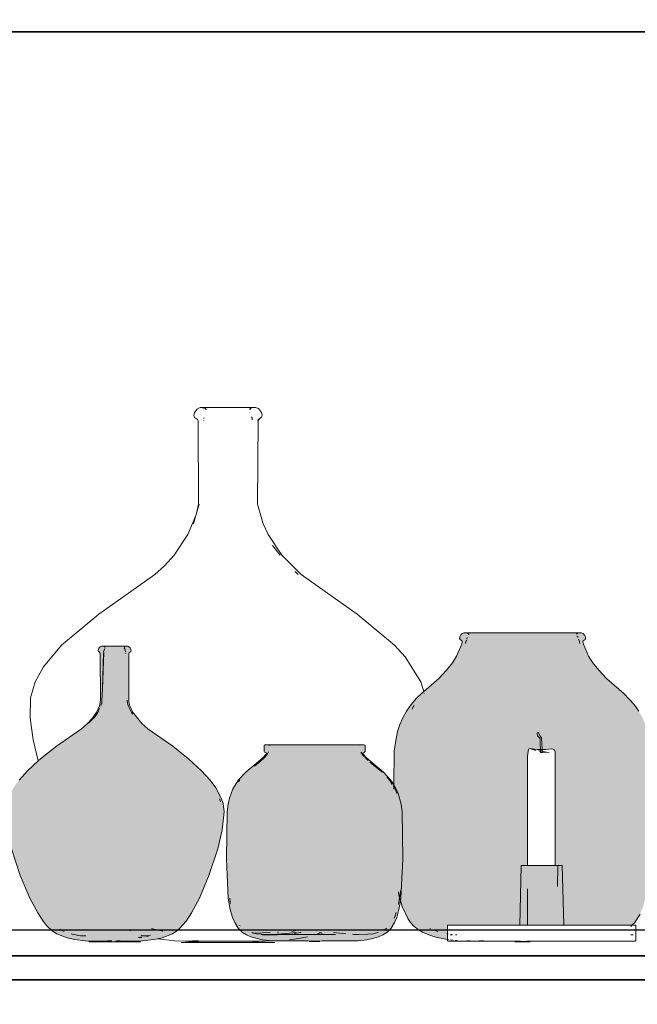
# Model space of a CAD drawing. Units: millimetres. Extents: x 446512 to 447461, y 70395 to 70610.
# Tile 16 of 39: x 446712 to 446725, y 70473 to 70493. Entities that reach past the tile are written whole.
import ezdxf

# ---------------------------------------------------------------- set-up
doc = ezdxf.new("R2010")
doc.units = ezdxf.units.MM
for name, color, linetype, lineweight in [('A-ANNO-DIMS', 2, 'Continuous', 18), ('A-FURN', 7, 'Continuous', 35), ('A-FURN-DECO', 8, 'Continuous', 13), ('A-FURN-PATT', 38, 'Continuous', 13)]:
    doc.layers.add(name, color=color, linetype=linetype, lineweight=lineweight)
doc.styles.get("Standard").update_dxf_attribs({"font": 'arial.ttf'})
doc.dimstyles.get("Standard").update_dxf_attribs({"dimtxt": 0.18, "dimasz": 0.18, "dimexe": 0.18, "dimexo": 0.0625, "dimgap": 0.09, "dimtad": 0, "dimtih": 1, "dimtoh": 1, "dimdec": 4, "dimzin": 0, "dimdsep": 46, "dimtxsty": 'Standard', "dimcen": 0.09, "dimadec": 0, "dimazin": 0, "dimtfac": 1, "dimtdec": 4, "dimtofl": 0, "dimtmove": 0, "dimatfit": 3, "dimfxl": 1, "dimtolj": 1, "dimtzin": 0, "dimarcsym": 0})

# ---------------------------------------------------------------- blocks, each defined once
blk = doc.blocks.new('*D32')
at = {"layer": 'A-ANNO-DIMS', "color": 0, "lineweight": -2, "transparency": 16777216}
for p, q in [((446730.76, 70474.405), (446678.043, 70474.405)), ((446678.223, 70474.225), (446678.223, 70474.075)), ((446678.223, 70473.562), (446678.223, 70473.711)), ((446728.946, 70473.382), (446678.043, 70473.382))]:
    blk.add_line(p, q, dxfattribs=at)
at = {"layer": 'A-ANNO-DIMS', "color": 0, "transparency": 16777216}
for points in [[(446678.193, 70474.225), (446678.253, 70474.225), (446678.223, 70474.405)], [(446678.193, 70473.562), (446678.253, 70473.562), (446678.223, 70473.382)]]:
    blk.add_solid(points, dxfattribs=at)
at = {"layer": 'Defpoints', "color": 0, "transparency": 16777216}
for p in [(446730.822, 70474.405), (446678.223, 70473.382), (446729.008, 70473.382)]:
    blk.add_point(p, dxfattribs=at)
at = {"layer": 'A-ANNO-DIMS', "color": 0, "transparency": 16777216, "insert": (446678.223, 70473.893), "char_height": 0.18, "attachment_point": 5}
blk.add_mtext('\\A1;1.02', dxfattribs=at)

msp = doc.modelspace()

# ---------------------------------------------------------------- hatches: boundary and pattern name
at = {"layer": 'A-FURN-PATT'}
h = msp.add_hatch(color=256, dxfattribs=at)
h.dxf.hatch_style = 1
h.paths.add_polyline_path([(446703.5722, 70477.5476), (446703.5295, 70477.5904), (446703.508, 70477.5904), (446703.383, 70477.6041), (446703.3062, 70477.6039), (446702.8621, 70477.6193), (446702.7177, 70477.6193), (446702.6174, 70477.6163), (446702.576, 70477.615), (446702.5757, 70477.6192), (446702.3373, 70477.6192), (446701.7238, 70477.5898), (446701.6039, 70477.5792), (446701.5612, 70477.5357), (446701.547, 70474.1653), (446703.5225, 70474.1653), (446703.5865, 70474.1653), (446703.5861, 70474.2632), (446703.5852, 70474.4594)])
h.paths.add_polyline_path([(446715.9764, 70475.5286), (446716.1565, 70476.0766), (446716.2492, 70476.4728), (446716.2873, 70476.8422), (446716.2666, 70477.0104), (446716.236, 70477.1061), (446716.1173, 70477.332), (446715.9979, 70477.4937), (446715.8249, 70477.6853), (446715.558, 70477.9316), (446715.2321, 70478.1882), (446714.7182, 70478.5467), (446714.5954, 70478.6535), (446714.3996, 70478.8999), (446714.3461, 70479.0185), (446714.3253, 70479.1028), (446714.3286, 70480.1095), (446714.368, 70480.1364), (446714.3744, 70480.152), (446714.3709, 70480.1808), (446714.3551, 70480.2131), (446714.3271, 70480.2359), (446714.3039, 70480.2478), (446714.2782, 70480.2478), (446714.259, 70480.2458), (446714.2432, 70480.2391), (446714.2375, 70480.2284), (446714.2369, 70480.2218), (446714.2301, 70480.2478), (446713.8255, 70480.2478), (446713.8277, 70480.2375), (446713.8104, 70480.2458), (446713.7912, 70480.2478), (446713.7655, 70480.2478), (446713.738, 70480.2359), (446713.7079, 70480.2028), (446713.6947, 70480.1567), (446713.6986, 70480.1448), (446713.717, 70480.1274), (446713.7341, 70480.1112), (446713.7407, 70480.1049), (446713.7473, 70479.1348), (446713.7233, 70479.0185), (446713.6698, 70478.8999), (446713.5684, 70478.7546), (446713.4739, 70478.6535), (446713.3511, 70478.5467), (446712.8373, 70478.1882), (446712.5114, 70477.9316), (446712.4629, 70477.8868), (446712.2445, 70477.6853), (446712.0714, 70477.4937), (446711.9521, 70477.332), (446711.866, 70477.1682), (446711.8333, 70477.1061), (446711.7899, 70476.9473), (446711.7821, 70476.8422), (446711.8202, 70476.4728), (446711.8563, 70476.3184), (446711.9128, 70476.0766), (446712.093, 70475.5286), (446712.2916, 70475.0627), (446712.4529, 70474.7607), (446712.5622, 70474.5947), (446712.6434, 70474.4935), (446712.7522, 70474.3925), (446712.8451, 70474.3334), (446713.0597, 70474.2483), (446713.2189, 70474.2124), (446713.4296, 70474.1861), (446713.8128, 70474.1834), (446713.5915, 70474.1683), (446714.5392, 70474.1683), (446714.4414, 70474.1779), (446714.1836, 70474.1834), (446714.6098, 70474.1861), (446714.8353, 70474.2124), (446714.9266, 70474.2312), (446715.0097, 70474.2483), (446715.2243, 70474.3334), (446715.3172, 70474.3925), (446715.3727, 70474.4388), (446715.5072, 70474.5947), (446715.6164, 70474.7607), (446715.7778, 70475.0627)])
h.paths.add_polyline_path([(446719.9646, 70475.8685), (446719.9469, 70476.8426), (446719.9277, 70476.9944), (446719.8688, 70477.2155), (446719.7757, 70477.4048), (446719.7115, 70477.4967), (446719.566, 70477.6531), (446719.2165, 70477.9493), (446719.1289, 70478.0481), (446719.1777, 70478.067), (446719.1866, 70478.0815), (446719.1867, 70478.209), (446719.1598, 70478.218), (446719.1369, 70478.2173), (446719.1374, 70478.2174), (446719.0341, 70478.2174), (446718.8666, 70478.218), (446718.6447, 70478.218), (446718.418, 70478.2174), (446718.1448, 70478.2174), (446717.8911, 70478.218), (446717.8873, 70478.218), (446717.6401, 70478.2174), (446717.4215, 70478.2174), (446717.2754, 70478.218), (446717.1987, 70478.218), (446717.2097, 70478.2113), (446717.1243, 70478.2174), (446717.1135, 70478.2124), (446717.1091, 70478.2029), (446717.1111, 70478.0815), (446717.1185, 70478.0683), (446717.1615, 70478.0517), (446717.1433, 70478.0167), (446717.0812, 70477.9493), (446716.7317, 70477.6531), (446716.5862, 70477.4967), (446716.47, 70477.311), (446716.3975, 70477.1183), (446716.37, 70476.9944), (446716.3508, 70476.8426), (446716.3331, 70475.8685), (446716.374, 70475.0624), (446716.4146, 70474.8322), (446716.4608, 70474.6687), (446716.5046, 70474.5619), (446716.5765, 70474.4449), (446716.6659, 70474.36), (446716.7457, 70474.3103), (446716.8351, 70474.2702), (446717.0729, 70474.2085), (446717.2886, 70474.1864), (446717.3803, 70474.1864), (446717.4428, 70474.1846), (446717.4556, 70474.1862), (446718.0146, 70474.1842), (446718.1072, 70474.1795), (446718.1371, 70474.1802), (446718.1473, 70474.1804), (446718.1566, 70474.1797), (446718.1569, 70474.1797), (446718.1592, 70474.1795), (446718.303, 70474.1842), (446719.0393, 70474.1865), (446719.2248, 70474.2085), (446719.365, 70474.2387), (446719.4626, 70474.2702), (446719.552, 70474.3103), (446719.6318, 70474.36), (446719.7212, 70474.4449), (446719.7931, 70474.5619), (446719.8369, 70474.6687), (446719.8831, 70474.8322), (446719.9155, 70475.0156), (446719.9237, 70475.0624)])
h.paths.add_polyline_path([(446718.18, 70474.3158), (446717.2692, 70474.3158), (446717.2092, 70474.3107), (446717.3763, 70474.3107)], flags=16)
h.paths.add_polyline_path([(446717.572, 70474.3384), (446717.5676, 70474.3381), (446717.5691, 70474.3381)], flags=16)
h.paths.add_polyline_path([(446722.3965, 70475.7383), (446722.4453, 70475.7383), (446722.4564, 70475.7383), (446722.4729, 70475.7383), (446722.4785, 70475.7384), (446722.4797, 70475.7383), (446722.4831, 70475.7383), (446722.4841, 70475.7384), (446722.5211, 70475.7384), (446722.4906, 70475.7381), (446722.4906, 70475.7384), (446722.4864, 70475.7383), (446722.4853, 70475.7383), (446722.4831, 70475.7383), (446722.4819, 70475.7383), (446722.4797, 70475.7383), (446722.4618, 70475.7383), (446722.4401, 70475.7383), (446722.4015, 70475.7383), (446722.3964, 70475.7341), (446722.3682, 70474.5084), (446722.5299, 70474.5084), (446723.2721, 70474.5084), (446723.2439, 70475.7341), (446723.2391, 70475.7383), (446723.2067, 70475.7383), (446723.1904, 70475.7383), (446723.1824, 70475.7383), (446723.1499, 70475.7382), (446723.1499, 70475.7384), (446723.1407, 70475.7384), (446723.1819, 70475.7384), (446723.1732, 70475.7384), (446723.1824, 70475.7383), (446723.1957, 70475.7383), (446723.1982, 70475.7383), (446723.2002, 70475.7383), (446723.2067, 70475.7383), (446723.2439, 70475.7383), (446723.2721, 70474.5084), (446724.6768, 70474.5084), (446724.7369, 70474.5652), (446724.8426, 70474.7369), (446724.9068, 70474.8938), (446724.9747, 70475.1338), (446725.0344, 70475.4718), (446725.0943, 70476.6554), (446725.0683, 70478.0856), (446725.0402, 70478.3085), (446724.9998, 70478.4903), (446724.9537, 70478.6331), (446724.8934, 70478.7733), (446724.817, 70478.911), (446724.7228, 70479.046), (446724.5091, 70479.2756), (446724.1522, 70479.5853), (446723.9922, 70479.7544), (446723.8721, 70479.9071), (446723.7862, 70480.0401), (446723.6778, 70480.2901), (446723.6684, 70480.351), (446723.714, 70480.381), (446723.7245, 70480.398), (446723.7213, 70480.4391), (446723.7096, 70480.4663), (446723.6751, 70480.5056), (446723.6405, 70480.5215), (446723.5985, 70480.5218), (446723.5958, 70480.5218), (446722.1196, 70480.5215), (446721.2867, 70480.5218), (446721.2939, 70480.516), (446721.2184, 70480.5218), (446721.1844, 70480.5072), (446721.155, 70480.479), (446721.1354, 70480.4391), (446721.1312, 70480.4035), (446721.1408, 70480.3826), (446721.1891, 70480.3558), (446721.179, 70480.2901), (446721.0706, 70480.0401), (446720.9847, 70479.9071), (446720.8645, 70479.7544), (446720.7046, 70479.5853), (446720.3925, 70479.3145), (446720.3476, 70479.2756), (446720.248, 70479.1783), (446720.134, 70479.046), (446720.0397, 70478.911), (446719.9634, 70478.7733), (446719.9031, 70478.6331), (446719.857, 70478.4903), (446719.8165, 70478.3085), (446719.7884, 70478.0856), (446719.7757, 70477.4048), (446719.8688, 70477.2155), (446719.9277, 70476.9944), (446719.9469, 70476.8426), (446719.9646, 70475.8685), (446719.9237, 70475.0624), (446719.9155, 70475.0156), (446719.9499, 70474.8938), (446720.064, 70474.6452), (446720.1198, 70474.5652), (446720.1819, 70474.4977), (446720.2884, 70474.4145), (446720.3682, 70474.3675), (446720.4995, 70474.3087), (446720.6428, 70474.2625), (446720.8486, 70474.2181), (446720.8834, 70474.214), (446720.8836, 70474.3337), (446720.8838, 70474.5084), (446722.3682, 70474.5084)])
h.paths.add_polyline_path([(446722.5299, 70477.9863), (446722.5458, 70478.1272), (446722.5844, 70478.1453), (446722.7245, 70478.1193), (446722.7937, 70478.1192), (446722.7905, 70478.2404), (446722.7882, 70478.3461), (446722.7354, 70478.4044), (446722.7276, 70478.4661), (446722.759, 70478.4678), (446722.7662, 70478.4254), (446722.8155, 70478.3594), (446722.8317, 70478.1191), (446722.9042, 70478.119), (446723.0314, 70478.1383), (446723.0829, 70478.1185), (446723.0949, 70478.0727), (446723.0974, 70475.7384), (446723.1135, 70475.7383), (446723.104, 70475.7384), (446723.1025, 70475.7384), (446723.0987, 70475.7384), (446723.0974, 70475.7383), (446723.0719, 70475.7383), (446723.018, 70475.7384), (446723.0095, 70475.7382), (446722.9885, 70475.7384), (446722.9576, 70475.7383), (446722.9328, 70475.7384), (446722.9244, 70475.7383), (446722.8841, 70475.7383), (446722.8055, 70475.7384), (446722.802, 70475.7383), (446722.7415, 70475.7384), (446722.7206, 70475.7383), (446722.7104, 70475.7384), (446722.6518, 70475.7384), (446722.6431, 70475.7383), (446722.6067, 70475.7383), (446722.5537, 70475.7384), (446722.5299, 70475.7383)], flags=16)
h.paths.add_polyline_path([(446722.7937, 70478.1192), (446722.8317, 70478.1191), (446722.8336, 70478.0906), (446722.8358, 70478.0578), (446722.7952, 70478.0599), (446722.7946, 70478.0859)], flags=0)
h.paths.add_polyline_path([(446723.5789, 70480.5193), (446723.5569, 70480.5185), (446723.5487, 70480.509)], flags=16)

# ---------------------------------------------------------------- linework, layer by layer
at = {"layer": 'A-FURN'}
msp.add_line((446686.5728, 70473.3815), (446746.5728, 70473.3815), dxfattribs=at)
for points in [[(446686.5728, 70493.3815), (446729.0084, 70493.3815), (446729.0084, 70473.3815), (446686.5728, 70473.3815)], [(446687.0728, 70492.8815), (446728.5084, 70492.8815), (446728.5084, 70473.8815), (446687.0728, 70473.8815)], [(446699.4288, 70473.3815), (446746.5728, 70473.3815), (446746.5728, 70453.3815), (446699.4288, 70453.3815)]]:
    msp.add_lwpolyline(points, close=True, dxfattribs=at)
at = {"layer": 'A-FURN-DECO'}
for p, q in [((446715.6813, 70485.0529), (446715.6671, 70484.9892)), ((446715.6792, 70484.9524), (446715.6671, 70484.9892)), ((446715.6813, 70485.0529), (446715.7339, 70485.1248)), ((446715.7952, 70485.1539), (446715.7339, 70485.1248)), ((446715.7952, 70485.1539), (446715.8037, 70485.1539)), ((446715.8037, 70485.1539), (446715.905, 70485.1381)), ((446715.8037, 70485.1539), (446716.0448, 70485.1539)), ((446715.905, 70485.1381), (446715.9182, 70485.1136)), ((446715.9182, 70485.1136), (446715.9181, 70485.1086)), ((446716.1174, 70485.1534), (446716.0448, 70485.1539)), ((446716.1788, 70485.1539), (446716.1174, 70485.1534)), ((446716.4113, 70485.1534), (446716.1788, 70485.1539)), ((446716.4755, 70485.1539), (446716.4113, 70485.1534)), ((446716.9331, 70485.1539), (446716.4755, 70485.1539)), ((446716.8532, 70485.1504), (446716.8127, 70485.143)), ((446716.8127, 70485.143), (446716.8448, 70485.146)), ((446716.8348, 70485.1407), (446716.8185, 70485.1136)), ((446716.8185, 70485.1136), (446716.8186, 70485.1102)), ((446716.8448, 70485.146), (446716.8348, 70485.1407)), ((446716.8448, 70485.146), (446716.9331, 70485.1539)), ((446716.8532, 70485.1504), (446716.8448, 70485.146)), ((446716.9913, 70485.1325), (446716.9331, 70485.1539)), ((446717.0554, 70485.0529), (446716.9913, 70485.1325)), ((446717.0691, 70485.003), (446717.0554, 70485.0529)), ((446717.0575, 70484.9524), (446717.0691, 70485.003)), ((446715.6792, 70484.9524), (446715.7414, 70484.91)), ((446715.7507, 70484.8843), (446715.7414, 70484.91)), ((446715.7625, 70483.1654), (446715.7507, 70484.8843)), ((446715.8712, 70484.8944), (446715.871, 70484.888)), ((446715.8727, 70484.9389), (446715.8723, 70484.9287)), ((446715.8776, 70484.9524), (446715.8727, 70484.9389)), ((446716.85, 70484.9623), (446716.857, 70484.9389)), ((446716.8641, 70484.9389), (446716.8559, 70484.9617)), ((446716.8652, 70484.9033), (446716.8641, 70484.9389)), ((446716.9864, 70484.888), (446716.9743, 70483.1654)), ((446717.01, 70484.9249), (446716.9771, 70484.888)), ((446716.9771, 70484.888), (446716.9998, 70484.9089)), ((446716.9864, 70484.888), (446716.9998, 70484.9089)), ((446716.9998, 70484.9089), (446717.0292, 70484.936)), ((446716.9998, 70484.9089), (446717.01, 70484.9249)), ((446717.0417, 70484.9475), (446717.01, 70484.9249)), ((446717.01, 70484.9249), (446717.0292, 70484.936)), ((446717.0292, 70484.936), (446717.0575, 70484.9524)), ((446717.0292, 70484.936), (446717.0417, 70484.9475)), ((446715.7194, 70482.9812), (446715.7625, 70483.1654)), ((446715.7715, 70483.1654), (446715.7194, 70482.9812)), ((446716.9743, 70483.1654), (446717.0904, 70482.7654)), ((446715.7194, 70482.9812), (446715.707, 70482.9375)), ((446715.5424, 70482.5434), (446715.707, 70482.9375)), ((446715.707, 70482.9375), (446715.6583, 70482.7654)), ((446717.1944, 70482.5434), (446717.0904, 70482.7654)), ((446715.2612, 70482.1197), (446715.5424, 70482.5434)), ((446717.4756, 70482.1197), (446717.1944, 70482.5434)), ((446717.2655, 70482.3446), (446717.2646, 70482.3458)), ((446717.441, 70482.1197), (446717.2848, 70482.3199)), ((446715.0599, 70481.8969), (446715.2612, 70482.1197)), ((446717.8715, 70481.7195), (446717.4756, 70482.1197)), ((446714.8653, 70481.7195), (446715.0599, 70481.8969)), ((446717.8097, 70481.7195), (446717.7467, 70481.78)), ((446713.7133, 70480.903), (446714.8653, 70481.7195)), ((446719.0235, 70480.903), (446717.8715, 70481.7195)), ((446713.7133, 70480.903), (446712.9441, 70480.267)), ((446719.7926, 70480.267), (446719.0235, 70480.903)), ((446721.1312, 70480.4035), (446721.1354, 70480.4391)), ((446721.1312, 70480.4035), (446721.1408, 70480.3826)), ((446721.1354, 70480.4391), (446721.155, 70480.479)), ((446721.1715, 70480.3655), (446721.1408, 70480.3826)), ((446721.155, 70480.479), (446721.1844, 70480.5072)), ((446721.1872, 70480.3435), (446721.1715, 70480.3655)), ((446721.179, 70480.2901), (446721.1872, 70480.3435)), ((446721.1844, 70480.5072), (446721.2184, 70480.5218)), ((446721.2184, 70480.5218), (446721.2939, 70480.516)), ((446721.2184, 70480.5218), (446722.1102, 70480.5218)), ((446721.2606, 70480.3384), (446721.2541, 70480.3026)), ((446721.2713, 70480.3708), (446721.2606, 70480.3384)), ((446721.2896, 70480.4263), (446721.2779, 70480.391)), ((446721.2939, 70480.516), (446721.3218, 70480.4931)), ((446721.3218, 70480.4931), (446721.3239, 70480.4799)), ((446722.1196, 70480.5215), (446722.1102, 70480.5218)), ((446722.1196, 70480.5215), (446723.5958, 70480.5218)), ((446723.5312, 70480.5176), (446723.5789, 70480.5193)), ((446723.5487, 70480.509), (446723.5356, 70480.4938)), ((446723.5432, 70480.4529), (446723.562, 70480.4386)), ((446723.5789, 70480.5193), (446723.5487, 70480.509)), ((446723.562, 70480.4386), (446723.5665, 70480.4257)), ((446723.5776, 70480.3943), (446723.5799, 70480.3876)), ((446723.5958, 70480.5218), (446723.5789, 70480.5193)), ((446723.5835, 70480.3773), (446723.5967, 70480.3398)), ((446723.5985, 70480.5218), (446723.5958, 70480.5218)), ((446723.5967, 70480.3398), (446723.6032, 70480.3017)), ((446723.5985, 70480.5218), (446723.6405, 70480.5215)), ((446723.6751, 70480.5056), (446723.6405, 70480.5215)), ((446723.6696, 70480.3435), (446723.6752, 70480.3554)), ((446723.6778, 70480.2901), (446723.6696, 70480.3435)), ((446723.7096, 70480.4663), (446723.6751, 70480.5056)), ((446723.6752, 70480.3554), (446723.714, 70480.381)), ((446723.7213, 70480.4391), (446723.7096, 70480.4663)), ((446723.714, 70480.381), (446723.7245, 70480.398)), ((446723.7245, 70480.398), (446723.7213, 70480.4391)), ((446712.5716, 70479.8256), (446712.9441, 70480.267)), ((446713.7079, 70480.2028), (446713.6947, 70480.1567)), ((446713.6947, 70480.1567), (446713.7014, 70480.1364)), ((446713.717, 70480.1274), (446713.7014, 70480.1364)), ((446713.704, 70480.1397), (446713.717, 70480.1274)), ((446713.738, 70480.2359), (446713.7079, 70480.2028)), ((446713.717, 70480.1274), (446713.7341, 70480.1112)), ((446713.7655, 70480.2478), (446713.738, 70480.2359)), ((446713.7912, 70480.2478), (446713.7655, 70480.2478)), ((446713.8104, 70480.2458), (446713.7912, 70480.2478)), ((446713.809, 70480.1312), (446713.8323, 70480.2016)), ((446713.8104, 70480.2458), (446713.8119, 70480.2478)), ((446713.8104, 70480.2458), (446713.8277, 70480.2375)), ((446713.8119, 70480.2478), (446714.2575, 70480.2478)), ((446713.8317, 70480.2185), (446713.8277, 70480.2375)), ((446714.2369, 70480.2218), (446714.2345, 70480.1967)), ((446714.2359, 70480.2255), (446714.2375, 70480.2284)), ((446714.2369, 70480.2218), (446714.2359, 70480.2255)), ((446714.2441, 70480.1941), (446714.2369, 70480.2218)), ((446714.239, 70480.2375), (446714.2374, 70480.2313)), ((446714.239, 70480.2312), (446714.2432, 70480.2391)), ((446714.259, 70480.2458), (446714.2432, 70480.2391)), ((446714.2602, 70480.1321), (446714.2453, 70480.1892)), ((446714.2575, 70480.2478), (446714.259, 70480.2458)), ((446714.2782, 70480.2478), (446714.259, 70480.2458)), ((446714.2605, 70480.1232), (446714.2602, 70480.1321)), ((446714.3039, 70480.2478), (446714.2782, 70480.2478)), ((446714.3271, 70480.2359), (446714.3039, 70480.2478)), ((446714.3271, 70480.2359), (446714.3551, 70480.2131)), ((446714.3337, 70480.113), (446714.368, 70480.1364)), ((446714.3709, 70480.1808), (446714.3551, 70480.2131)), ((446714.368, 70480.1364), (446714.3744, 70480.152)), ((446714.3709, 70480.1808), (446714.3744, 70480.152)), ((446720.015, 70480.0256), (446719.7926, 70480.267)), ((446721.0706, 70480.0401), (446721.179, 70480.2901)), ((446723.7862, 70480.0401), (446723.6778, 70480.2901)), ((446713.7341, 70480.1112), (446713.7407, 70480.1008)), ((446713.7341, 70480.1112), (446713.745, 70480.1008)), ((446713.7407, 70480.1008), (446713.7473, 70479.1348)), ((446713.7828, 70479.3698), (446713.8079, 70480.1173)), ((446713.7828, 70479.3698), (446713.8109, 70480.1165)), ((446714.2613, 70480.0995), (446714.2611, 70480.105)), ((446714.3285, 70480.0988), (446714.3253, 70479.1028)), ((446714.3285, 70480.0988), (446714.3337, 70480.113)), ((446720.015, 70480.0256), (446720.336, 70479.5124)), ((446720.9847, 70479.9071), (446721.0706, 70480.0401)), ((446723.8721, 70479.9071), (446723.7862, 70480.0401)), ((446712.4008, 70479.5124), (446712.5716, 70479.8256)), ((446720.7046, 70479.5853), (446720.8645, 70479.7544)), ((446720.8645, 70479.7544), (446720.9847, 70479.9071)), ((446723.9922, 70479.7544), (446723.8721, 70479.9071)), ((446724.1522, 70479.5853), (446723.9922, 70479.7544)), ((446720.3925, 70479.3145), (446720.7046, 70479.5853)), ((446724.5091, 70479.2756), (446724.1522, 70479.5853)), ((446712.4008, 70479.5124), (446712.3062, 70479.1812)), ((446713.7828, 70479.3698), (446713.7738, 70479.1282)), ((446720.3925, 70479.3145), (446720.336, 70479.5124)), ((446720.3476, 70479.2756), (446720.3925, 70479.3145)), ((446712.3062, 70479.1812), (446712.3006, 70478.765)), ((446713.7473, 70479.1348), (446713.7233, 70479.0185)), ((446713.7738, 70479.1282), (446713.7739, 70479.1027)), ((446714.294, 70479.1169), (446714.2934, 70479.1348)), ((446714.3157, 70479.0226), (446714.294, 70479.1169)), ((446720.134, 70479.046), (446720.248, 70479.1783)), ((446720.248, 70479.1783), (446720.3476, 70479.2756)), ((446720.4059, 70479.2674), (446720.4036, 70479.2756)), ((446724.7228, 70479.046), (446724.5091, 70479.2756)), ((446713.6698, 70478.8999), (446713.7233, 70479.0185)), ((446713.7258, 70478.963), (446713.6893, 70478.8849)), ((446713.7532, 70479.0214), (446713.7492, 70479.013)), ((446713.7726, 70479.0977), (446713.7571, 70479.0359)), ((446713.7716, 70479.0708), (446713.7726, 70479.0977)), ((446713.7739, 70479.1027), (446713.7726, 70479.0977)), ((446714.3801, 70478.8849), (446714.3157, 70479.0226)), ((446714.3253, 70479.1028), (446714.3461, 70479.0185)), ((446714.3461, 70479.0185), (446714.3996, 70478.8999)), ((446720.0397, 70478.911), (446719.9634, 70478.7733)), ((446720.134, 70479.046), (446720.0397, 70478.911)), ((446720.1787, 70478.9969), (446720.1524, 70478.9541)), ((446720.1995, 70479.0239), (446720.1787, 70478.9969)), ((446724.817, 70478.911), (446724.7228, 70479.046)), ((446712.361, 70478.3226), (446712.3006, 70478.765)), ((446713.5684, 70478.7546), (446713.4739, 70478.6535)), ((446713.4976, 70478.6643), (446713.6325, 70478.7994)), ((446713.5684, 70478.7546), (446713.6698, 70478.8999)), ((446713.6893, 70478.8849), (446713.6325, 70478.7994)), ((446714.4095, 70478.8455), (446714.3801, 70478.8849)), ((446714.3996, 70478.8999), (446714.5954, 70478.6535)), ((446719.9031, 70478.6331), (446719.9634, 70478.7733)), ((446713.3511, 70478.5467), (446712.8373, 70478.1882)), ((446713.4739, 70478.6535), (446713.3511, 70478.5467)), ((446714.7182, 70478.5467), (446714.5954, 70478.6535)), ((446715.2321, 70478.1882), (446714.7182, 70478.5467)), ((446719.857, 70478.4903), (446719.9031, 70478.6331)), ((446712.4629, 70477.8868), (446712.361, 70478.3226)), ((446719.7884, 70478.0856), (446719.8165, 70478.3085)), ((446719.8165, 70478.3085), (446719.857, 70478.4903)), ((446722.759, 70478.4678), (446722.7276, 70478.4661)), ((446722.7354, 70478.4044), (446722.7276, 70478.4661)), ((446722.7882, 70478.3461), (446722.7354, 70478.4044)), ((446722.7662, 70478.4254), (446722.759, 70478.4678)), ((446722.8155, 70478.3594), (446722.7662, 70478.4254)), ((446722.7905, 70478.2404), (446722.7882, 70478.3461)), ((446722.8155, 70478.3594), (446722.8317, 70478.1191)), ((446712.5114, 70477.9316), (446712.8373, 70478.1882)), ((446715.558, 70477.9316), (446715.2321, 70478.1882)), ((446717.1135, 70478.2124), (446717.1091, 70478.2029)), ((446717.1111, 70478.0815), (446717.1091, 70478.2029)), ((446717.1243, 70478.2174), (446717.1135, 70478.2124)), ((446717.1582, 70478.2174), (446717.1243, 70478.2174)), ((446717.1243, 70478.2174), (446717.2097, 70478.2113)), ((446717.1655, 70478.218), (446717.1582, 70478.2174)), ((446717.1655, 70478.218), (446717.2754, 70478.218)), ((446717.2097, 70478.2113), (446717.215, 70478.208)), ((446717.2097, 70478.2113), (446717.2382, 70478.2087)), ((446717.2382, 70478.2087), (446717.2396, 70478.2087)), ((446717.4215, 70478.2174), (446717.2754, 70478.218)), ((446717.4215, 70478.2174), (446717.6401, 70478.2174)), ((446717.6401, 70478.2174), (446717.8833, 70478.218)), ((446717.8873, 70478.218), (446717.8833, 70478.218)), ((446717.8873, 70478.218), (446717.8911, 70478.218)), ((446717.8911, 70478.218), (446718.1448, 70478.2174)), ((446718.418, 70478.2174), (446718.1448, 70478.2174)), ((446718.6508, 70478.218), (446718.418, 70478.2174)), ((446718.6619, 70478.218), (446718.6508, 70478.218)), ((446718.6619, 70478.218), (446718.8666, 70478.218)), ((446719.0341, 70478.2174), (446718.8666, 70478.218)), ((446719.1374, 70478.2174), (446719.0341, 70478.2174)), ((446719.082, 70478.2081), (446719.1374, 70478.2174)), ((446719.1395, 70478.2174), (446719.1374, 70478.2174)), ((446719.1395, 70478.2174), (446719.1598, 70478.218)), ((446719.1598, 70478.218), (446719.1867, 70478.209)), ((446719.1867, 70478.209), (446719.1866, 70478.0815)), ((446722.5299, 70477.9863), (446722.5458, 70478.1272)), ((446722.5844, 70478.1453), (446722.5458, 70478.1272)), ((446722.7245, 70478.1193), (446722.5844, 70478.1453)), ((446722.6965, 70478.1045), (446722.5974, 70478.1356)), ((446722.5974, 70478.1356), (446722.7245, 70478.1193)), ((446722.7245, 70478.1193), (446722.7937, 70478.1192)), ((446722.7942, 70478.1007), (446722.7245, 70478.1193)), ((446722.7937, 70478.1192), (446722.7905, 70478.2404)), ((446722.7942, 70478.1007), (446722.7937, 70478.1192)), ((446722.7937, 70478.1192), (446722.8317, 70478.1191)), ((446722.8336, 70478.0906), (446722.7942, 70478.1007)), ((446722.7943, 70478.0946), (446722.7942, 70478.0982)), ((446722.8317, 70478.1191), (446722.8336, 70478.0906)), ((446722.8317, 70478.1191), (446722.9042, 70478.119)), ((446722.9042, 70478.119), (446723.0314, 70478.1383)), ((446723.0314, 70478.1383), (446723.0829, 70478.1185)), ((446723.0949, 70478.0727), (446723.0829, 70478.1185)), ((446712.4629, 70477.8868), (446712.5114, 70477.9316)), ((446715.8249, 70477.6853), (446715.558, 70477.9316)), ((446717.0812, 70477.9493), (446716.7317, 70477.6531)), ((446717.0262, 70477.8746), (446717.1225, 70477.9672)), ((446717.1433, 70478.0167), (446717.0812, 70477.9493)), ((446717.1111, 70478.0815), (446717.1185, 70478.0683)), ((446717.1185, 70478.0683), (446717.1519, 70478.0554)), ((446717.1777, 70478.0319), (446717.1225, 70477.9672)), ((446717.156, 70478.0411), (446717.1433, 70478.0167)), ((446717.1519, 70478.0554), (446717.156, 70478.0411)), ((446717.1777, 70478.0319), (446717.2018, 70478.0745)), ((446719.1645, 70477.9809), (446719.0965, 70478.0677)), ((446719.1443, 70478.0541), (446719.1412, 70478.0465)), ((446719.1412, 70478.0465), (446719.1481, 70478.0264)), ((446719.1777, 70478.067), (446719.1443, 70478.0541)), ((446719.1481, 70478.0264), (446719.2165, 70477.9493)), ((446719.1866, 70478.0815), (446719.1777, 70478.067)), ((446719.2498, 70477.8954), (446719.1793, 70477.9632)), ((446719.2165, 70477.9493), (446719.566, 70477.6531)), ((446719.7757, 70477.4048), (446719.7884, 70478.0856)), ((446722.5299, 70475.7383), (446722.5299, 70477.9863)), ((446722.7949, 70478.0737), (446722.7755, 70478.0797)), ((446722.7949, 70478.0737), (446722.7946, 70478.0859)), ((446722.8144, 70478.0676), (446722.7949, 70478.0737)), ((446722.7952, 70478.0599), (446722.7949, 70478.0737)), ((446722.8203, 70478.0586), (446722.7952, 70478.0599)), ((446722.8144, 70478.0676), (446722.8353, 70478.0658)), ((446722.8203, 70478.0586), (446722.8358, 70478.0582)), ((446722.9769, 70478.0539), (446722.8336, 70478.0906)), ((446722.8339, 70478.0856), (446722.8348, 70478.0729)), ((446722.8353, 70478.0658), (446722.8358, 70478.0582)), ((446722.8353, 70478.0658), (446722.9085, 70478.0597)), ((446723.0949, 70478.0727), (446723.0974, 70475.7383)), ((446712.2445, 70477.6853), (446712.4629, 70477.8868)), ((446716.911, 70477.7811), (446717.0262, 70477.8746)), ((446719.5332, 70477.6623), (446719.2866, 70477.8624)), ((446712.0714, 70477.4937), (446712.2445, 70477.6853)), ((446715.9979, 70477.4937), (446715.8249, 70477.6853)), ((446716.1173, 70477.332), (446715.9979, 70477.4937)), ((446716.5862, 70477.4967), (446716.47, 70477.311)), ((446716.7317, 70477.6531), (446716.5862, 70477.4967)), ((446716.6022, 70477.486), (446716.6112, 70477.4967)), ((446719.5425, 70477.6531), (446719.5332, 70477.6623)), ((446719.566, 70477.6531), (446719.7115, 70477.4967)), ((446719.6955, 70477.486), (446719.6342, 70477.5596)), ((446719.7115, 70477.4967), (446719.7757, 70477.4048)), ((446716.1173, 70477.332), (446716.236, 70477.1061)), ((446716.47, 70477.311), (446716.3975, 70477.1183)), ((446716.5831, 70477.4579), (446716.6022, 70477.486)), ((446719.7452, 70477.4048), (446719.6955, 70477.486)), ((446719.7739, 70477.3579), (446719.7757, 70477.4048)), ((446719.7752, 70477.3558), (446719.7739, 70477.3579)), ((446719.7743, 70477.3059), (446719.7752, 70477.3558)), ((446719.8107, 70477.2978), (446719.7752, 70477.3558)), ((446719.7757, 70477.4048), (446719.8688, 70477.2155)), ((446719.8413, 70477.2155), (446719.8107, 70477.2978)), ((446716.1925, 70477.1061), (446716.2108, 70477.0485)), ((446716.2666, 70477.0104), (446716.236, 70477.1061)), ((446716.3975, 70477.1183), (446716.37, 70476.9944)), ((446719.8688, 70477.2155), (446719.9277, 70476.9944)), ((446716.2873, 70476.8422), (446716.2666, 70477.0104)), ((446716.37, 70476.9944), (446716.3508, 70476.8426)), ((446719.9277, 70476.9944), (446719.9469, 70476.8426)), ((446716.2873, 70476.8422), (446716.2492, 70476.4728)), ((446716.3508, 70476.8426), (446716.3331, 70475.8685)), ((446719.9469, 70476.8426), (446719.9646, 70475.8685)), ((446716.2492, 70476.4728), (446716.1565, 70476.0766)), ((446712.093, 70475.5286), (446711.9128, 70476.0766)), ((446716.1565, 70476.0766), (446715.9764, 70475.5286)), ((446716.3331, 70475.8685), (446716.374, 70475.0624)), ((446719.9646, 70475.8685), (446719.9237, 70475.0624)), ((446722.3682, 70474.5084), (446722.3964, 70475.7341)), ((446722.3964, 70475.7341), (446722.4015, 70475.7383)), ((446722.4015, 70475.7383), (446722.438, 70475.7383)), ((446722.438, 70475.7383), (446722.4401, 70475.7383)), ((446722.4401, 70475.7383), (446722.4564, 70475.7383)), ((446722.4564, 70475.7383), (446722.4601, 70475.7383)), ((446722.4601, 70475.7383), (446722.4618, 70475.7383)), ((446722.4618, 70475.7383), (446722.4728, 70475.7383)), ((446722.4728, 70475.7383), (446722.4785, 70475.7384)), ((446722.4785, 70475.7384), (446722.4819, 70475.7383)), ((446722.4819, 70475.7383), (446722.4839, 70475.7384)), ((446722.4839, 70475.7384), (446722.4864, 70475.7383)), ((446722.4864, 70475.7383), (446722.4906, 70475.7384)), ((446722.4935, 70475.7384), (446722.4906, 70475.7384)), ((446722.4906, 70475.7384), (446722.4907, 70475.7341)), ((446722.4935, 70475.7384), (446722.4953, 70475.7384)), ((446722.4953, 70475.7384), (446722.5004, 70475.7384)), ((446722.5089, 70475.7384), (446722.5004, 70475.7384)), ((446722.5111, 70475.7383), (446722.5089, 70475.7384)), ((446722.5111, 70475.7383), (446722.519, 70475.7384)), ((446722.519, 70475.7384), (446722.5211, 70475.7384)), ((446722.5211, 70475.7384), (446722.5225, 70475.7384)), ((446722.5225, 70475.7384), (446722.5299, 70475.7383)), ((446722.5299, 70475.7341), (446722.5299, 70475.7383)), ((446722.5404, 70475.7383), (446722.5299, 70475.7383)), ((446722.5404, 70475.7383), (446722.5537, 70475.7384)), ((446722.5997, 70475.7384), (446722.5537, 70475.7384)), ((446722.6067, 70475.7383), (446722.5997, 70475.7384)), ((446722.6067, 70475.7383), (446722.6431, 70475.7383)), ((446722.6431, 70475.7383), (446722.6518, 70475.7384)), ((446722.6518, 70475.7384), (446722.7104, 70475.7384)), ((446722.7206, 70475.7383), (446722.7104, 70475.7384)), ((446722.7206, 70475.7383), (446722.7415, 70475.7384)), ((446722.802, 70475.7383), (446722.7415, 70475.7384)), ((446722.802, 70475.7383), (446722.8055, 70475.7384)), ((446722.8055, 70475.7384), (446722.8701, 70475.7384)), ((446722.8841, 70475.7383), (446722.8701, 70475.7384)), ((446722.8841, 70475.7383), (446722.9244, 70475.7383)), ((446722.9244, 70475.7383), (446722.9328, 70475.7384)), ((446722.9563, 70475.7383), (446722.9328, 70475.7384)), ((446722.9592, 70475.7383), (446722.9563, 70475.7383)), ((446722.9627, 70475.7384), (446722.9592, 70475.7383)), ((446722.9627, 70475.7384), (446722.9652, 70475.7383)), ((446722.9652, 70475.7383), (446722.9669, 70475.7383)), ((446722.9669, 70475.7383), (446722.9885, 70475.7384)), ((446722.9973, 70475.7383), (446722.9885, 70475.7384)), ((446723.0145, 70475.7383), (446722.9973, 70475.7383)), ((446723.0145, 70475.7383), (446723.018, 70475.7384)), ((446723.018, 70475.7384), (446723.0657, 70475.7384)), ((446723.0719, 70475.7383), (446723.0657, 70475.7384)), ((446723.0719, 70475.7383), (446723.0892, 70475.7383)), ((446723.0937, 70475.7383), (446723.0892, 70475.7383)), ((446723.0974, 70475.7383), (446723.0937, 70475.7383)), ((446723.0987, 70475.7384), (446723.0974, 70475.7383)), ((446723.0974, 70475.7383), (446723.0974, 70475.7341)), ((446723.1025, 70475.7384), (446723.0987, 70475.7384)), ((446723.104, 70475.7384), (446723.1025, 70475.7384)), ((446723.104, 70475.7384), (446723.1135, 70475.7383)), ((446723.1166, 70475.7383), (446723.1135, 70475.7383)), ((446723.1292, 70475.7383), (446723.1166, 70475.7383)), ((446723.1325, 70475.7383), (446723.1292, 70475.7383)), ((446723.1325, 70475.7383), (446723.1407, 70475.7384)), ((446723.1499, 70475.7384), (446723.1407, 70475.7384)), ((446723.1499, 70475.7384), (446723.1435, 70475.3041)), ((446723.1528, 70475.7384), (446723.1499, 70475.7384)), ((446723.1555, 70475.7383), (446723.1528, 70475.7384)), ((446723.1555, 70475.7383), (446723.1732, 70475.7384)), ((446723.1732, 70475.7384), (446723.177, 70475.7383)), ((446723.177, 70475.7383), (446723.1811, 70475.7383)), ((446723.1811, 70475.7383), (446723.1957, 70475.7383)), ((446723.1957, 70475.7383), (446723.1982, 70475.7383)), ((446723.1982, 70475.7383), (446723.2002, 70475.7383)), ((446723.2002, 70475.7383), (446723.2067, 70475.7383)), ((446723.2067, 70475.7383), (446723.2391, 70475.7383)), ((446723.2439, 70475.7341), (446723.2391, 70475.7383)), ((446723.2721, 70474.5084), (446723.2439, 70475.7341)), ((446712.093, 70475.5286), (446712.2916, 70475.0627)), ((446715.7778, 70475.0627), (446715.9764, 70475.5286)), ((446712.4529, 70474.7607), (446712.2916, 70475.0627)), ((446715.7778, 70475.0627), (446715.6164, 70474.7607)), ((446716.374, 70475.0624), (446716.4146, 70474.8322)), ((446716.4134, 70474.9835), (446716.402, 70475.0624)), ((446719.8821, 70475.1338), (446719.8714, 70475.1943)), ((446719.8979, 70475.0778), (446719.8821, 70475.1338)), ((446719.8843, 70474.9835), (446719.8979, 70475.0778)), ((446719.8979, 70475.0778), (446719.9198, 70475.229)), ((446719.9155, 70475.0156), (446719.8979, 70475.0778)), ((446719.9237, 70475.0624), (446719.9155, 70475.0156)), ((446722.5299, 70474.5084), (446722.5299, 70475.2593)), ((446716.4216, 70474.9543), (446716.4134, 70474.9835)), ((446719.8744, 70474.9421), (446719.8843, 70474.9835)), ((446719.9155, 70475.0156), (446719.8831, 70474.8322)), ((446719.9499, 70474.8938), (446719.9155, 70475.0156)), ((446720.064, 70474.6452), (446719.9499, 70474.8938)), ((446712.4529, 70474.7607), (446712.5622, 70474.5947)), ((446715.5072, 70474.5947), (446715.6164, 70474.7607)), ((446716.4146, 70474.8322), (446716.4608, 70474.6687)), ((446716.4608, 70474.6687), (446716.5046, 70474.5619)), ((446719.7824, 70474.6556), (446719.8053, 70474.6995)), ((446719.8369, 70474.6687), (446719.7931, 70474.5619)), ((446719.8053, 70474.6995), (446719.8298, 70474.772)), ((446719.8831, 70474.8322), (446719.8369, 70474.6687)), ((446724.7369, 70474.5652), (446724.8426, 70474.7369)), ((446712.6434, 70474.4935), (446712.5622, 70474.5947)), ((446712.7522, 70474.3925), (446712.6434, 70474.4935)), ((446715.3727, 70474.4388), (446715.5072, 70474.5947)), ((446716.5046, 70474.5619), (446716.5765, 70474.4449)), ((446716.619, 70474.4927), (446716.6062, 70474.5047)), ((446719.7931, 70474.5619), (446719.7212, 70474.4449)), ((446720.1198, 70474.5652), (446720.064, 70474.6452)), ((446720.1819, 70474.4977), (446720.1198, 70474.5652)), ((446720.2884, 70474.4145), (446720.1819, 70474.4977)), ((446720.8836, 70474.3337), (446720.8838, 70474.5084)), ((446722.3682, 70474.5084), (446720.8838, 70474.5084)), ((446722.5299, 70474.5084), (446722.3682, 70474.5084)), ((446722.5299, 70474.5084), (446723.2721, 70474.5084)), ((446724.6505, 70474.5084), (446723.2721, 70474.5084)), ((446724.6505, 70474.5084), (446724.6767, 70474.5083)), ((446724.6505, 70474.4831), (446724.6767, 70474.5083)), ((446724.6767, 70474.5083), (446724.7369, 70474.5652)), ((446724.685, 70474.5083), (446724.6767, 70474.5083)), ((446724.6957, 70474.5084), (446724.685, 70474.5083)), ((446724.6957, 70474.5084), (446724.7565, 70474.5084)), ((446724.757, 70474.1952), (446724.7565, 70474.5084)), ((446712.8451, 70474.3334), (446712.7522, 70474.3925)), ((446713.0597, 70474.2483), (446712.8451, 70474.3334)), ((446712.9446, 70474.4003), (446712.9085, 70474.4246)), ((446712.995, 70474.3823), (446712.9446, 70474.4003)), ((446713.1593, 70474.3238), (446713.1388, 70474.3311)), ((446713.3306, 70474.2923), (446713.1593, 70474.3238)), ((446713.4447, 70474.2879), (446713.3306, 70474.2923)), ((446714.3452, 70474.3997), (446714.3634, 70474.3925)), ((446714.5288, 70474.2558), (446714.5635, 70474.2558)), ((446714.5357, 70474.2567), (446714.5635, 70474.2558)), ((446714.5917, 70474.2558), (446714.5635, 70474.2558)), ((446714.6452, 70474.2886), (446714.571, 70474.2857)), ((446714.5898, 70474.3027), (446714.604, 70474.2971)), ((446714.604, 70474.2971), (446714.6452, 70474.2886)), ((446714.7388, 70474.2923), (446714.6452, 70474.2886)), ((446714.6452, 70474.2886), (446714.6593, 70474.2857)), ((446714.6972, 70474.2779), (446714.708, 70474.2757)), ((446714.7388, 70474.2923), (446714.7762, 70474.3009)), ((446714.8137, 70474.4337), (446714.7942, 70474.4388)), ((446714.8137, 70474.4337), (446715.0295, 70474.3857)), ((446715.2243, 70474.3334), (446715.0097, 70474.2483)), ((446715.2243, 70474.3334), (446715.3172, 70474.3925)), ((446715.3727, 70474.4388), (446715.3172, 70474.3925)), ((446716.5765, 70474.4449), (446716.6659, 70474.36)), ((446716.6659, 70474.36), (446716.7457, 70474.3103)), ((446716.7457, 70474.3103), (446716.8351, 70474.2702)), ((446716.8351, 70474.2702), (446717.0729, 70474.2085)), ((446716.8989, 70474.3472), (446716.8572, 70474.3586)), ((446716.8721, 70474.3461), (446716.8989, 70474.3472)), ((446716.8989, 70474.3472), (446717.2324, 70474.36)), ((446716.9465, 70474.3341), (446716.8989, 70474.3472)), ((446717.0513, 70474.3209), (446716.9465, 70474.3341)), ((446717.2092, 70474.3107), (446717.0481, 70474.316)), ((446717.2692, 70474.3158), (446717.0513, 70474.3209)), ((446717.0791, 70474.3107), (446717.2092, 70474.3107)), ((446717.3763, 70474.3107), (446717.2092, 70474.3107)), ((446717.5676, 70474.3381), (446717.2692, 70474.3158)), ((446717.2692, 70474.3158), (446718.18, 70474.3158)), ((446717.3863, 70474.3659), (446717.4086, 70474.3668)), ((446717.5676, 70474.3381), (446717.5691, 70474.3381)), ((446717.7637, 70474.36), (446717.5691, 70474.3381)), ((446717.6781, 70474.3794), (446717.7598, 70474.3992)), ((446717.862, 70474.36), (446717.7259, 70474.3381)), ((446717.7702, 70474.3607), (446717.768, 70474.3605)), ((446718.002, 70474.2702), (446717.8172, 70474.2322)), ((446717.862, 70474.36), (446717.8692, 70474.36)), ((446718.18, 70474.3158), (446718.166, 70474.3103)), ((446718.2698, 70474.3514), (446718.18, 70474.3158)), ((446718.5802, 70474.3158), (446718.18, 70474.3158)), ((446718.2698, 70474.3514), (446718.2494, 70474.36)), ((446718.2567, 70474.36), (446718.2698, 70474.3514)), ((446718.2698, 70474.3514), (446718.2722, 70474.3524)), ((446718.2914, 70474.36), (446718.2722, 70474.3524)), ((446718.2722, 70474.3524), (446718.3017, 70474.3381)), ((446718.5367, 70474.36), (446718.7286, 70474.3381)), ((446718.7286, 70474.3381), (446718.7885, 70474.3341)), ((446718.9315, 70474.3245), (446719.0605, 70474.3158)), ((446719.0605, 70474.3158), (446718.9554, 70474.3158)), ((446719.0605, 70474.3158), (446719.2464, 70474.3209)), ((446719.2464, 70474.3209), (446719.3512, 70474.3341)), ((446719.3512, 70474.3341), (446719.4489, 70474.3566)), ((446719.4626, 70474.2702), (446719.365, 70474.2387)), ((446719.4489, 70474.3566), (446719.4562, 70474.36)), ((446719.552, 70474.3103), (446719.4626, 70474.2702)), ((446719.5479, 70474.4026), (446719.617, 70474.4348)), ((446719.6318, 70474.36), (446719.552, 70474.3103)), ((446719.617, 70474.4348), (446719.6295, 70474.4449)), ((446719.7212, 70474.4449), (446719.6318, 70474.36)), ((446720.3682, 70474.3675), (446720.2884, 70474.4145)), ((446720.4995, 70474.3087), (446720.3682, 70474.3675)), ((446720.6428, 70474.2625), (446720.4995, 70474.3087)), ((446720.5163, 70474.4405), (446720.5355, 70474.4328)), ((446720.5852, 70474.4128), (446720.6248, 70474.3969)), ((446720.6248, 70474.3969), (446720.687, 70474.379)), ((446720.8486, 70474.2181), (446720.6428, 70474.2625)), ((446720.8658, 70474.3371), (446720.8836, 70474.3337)), ((446720.8834, 70474.214), (446720.8836, 70474.3337)), ((446720.8836, 70474.3337), (446720.8967, 70474.3312)), ((446720.9443, 70474.3222), (446720.9727, 70474.3168)), ((446720.9443, 70474.3123), (446720.9533, 70474.3123)), ((446720.9533, 70474.3123), (446720.9799, 70474.3121)), ((446720.9727, 70474.3168), (446720.9791, 70474.3165)), ((446721.0473, 70474.3141), (446721.0755, 70474.3131)), ((446721.0478, 70474.3117), (446721.0755, 70474.3115)), ((446724.6871, 70474.3123), (446724.6508, 70474.3121)), ((446724.7044, 70474.3123), (446724.6871, 70474.3123)), ((446713.2189, 70474.2124), (446713.0597, 70474.2483)), ((446713.4296, 70474.1861), (446713.2189, 70474.2124)), ((446713.4296, 70474.1861), (446713.8128, 70474.1834)), ((446713.5915, 70474.1683), (446713.5034, 70474.1683)), ((446713.8128, 70474.1834), (446713.5915, 70474.1683)), ((446714.5392, 70474.1683), (446713.5915, 70474.1683)), ((446713.8128, 70474.1834), (446713.8867, 70474.1842)), ((446713.8867, 70474.1842), (446713.9461, 70474.1839)), ((446713.9461, 70474.1839), (446713.9755, 70474.184)), ((446713.9776, 70474.184), (446713.9755, 70474.184)), ((446714.0498, 70474.1834), (446714.0864, 70474.1844)), ((446714.152, 70474.1842), (446714.0864, 70474.1844)), ((446714.152, 70474.1842), (446714.1836, 70474.1834)), ((446714.1836, 70474.1834), (446714.6098, 70474.1861)), ((446714.4414, 70474.1779), (446714.1836, 70474.1834)), ((446714.5392, 70474.1683), (446714.4414, 70474.1779)), ((446714.566, 70474.1683), (446714.5392, 70474.1683)), ((446714.8353, 70474.2124), (446714.6098, 70474.1861)), ((446714.9266, 70474.2312), (446714.8353, 70474.2124)), ((446714.9197, 70474.2321), (446714.9266, 70474.2312)), ((446715.0097, 70474.2483), (446714.9266, 70474.2312)), ((446714.9266, 70474.2312), (446715.2734, 70474.1846)), ((446715.96, 70474.1797), (446715.2734, 70474.1846)), ((446715.4069, 70474.1523), (446715.4238, 70474.1523)), ((446715.4238, 70474.1523), (446715.5489, 70474.1696)), ((446715.4238, 70474.1523), (446717.2813, 70474.1523)), ((446715.96, 70474.1797), (446715.5489, 70474.1696)), ((446715.7646, 70474.1846), (446715.6401, 70474.1846)), ((446715.8384, 70474.1827), (446715.7646, 70474.1846)), ((446715.8384, 70474.1827), (446715.96, 70474.1797)), ((446715.9632, 70474.1823), (446715.8384, 70474.1827)), ((446715.96, 70474.1797), (446716.2027, 70474.1807)), ((446716.2027, 70474.1807), (446715.9632, 70474.1823)), ((446716.2027, 70474.1807), (446716.2188, 70474.1806)), ((446716.2188, 70474.1806), (446716.3251, 70474.1812)), ((446716.3251, 70474.1812), (446716.3411, 70474.1797)), ((446716.3631, 70474.181), (446716.3411, 70474.1797)), ((446716.3819, 70474.1814), (446716.3631, 70474.181)), ((446716.397, 70474.1813), (446716.3819, 70474.1814)), ((446716.4054, 70474.1815), (446716.397, 70474.1813)), ((446716.4197, 70474.1812), (446716.4054, 70474.1815)), ((446716.4427, 70474.1813), (446716.4197, 70474.1812)), ((446716.4961, 70474.1806), (446716.4427, 70474.1813)), ((446716.4961, 70474.1806), (446716.5372, 70474.1808)), ((446716.8494, 70474.1826), (446716.5372, 70474.1808)), ((446716.7699, 70474.1797), (446716.5372, 70474.1808)), ((446716.7699, 70474.1797), (446716.8494, 70474.1826)), ((446716.7699, 70474.1797), (446716.985, 70474.1696)), ((446717.1886, 70474.1846), (446716.8494, 70474.1826)), ((446716.985, 70474.1696), (446717.2813, 70474.1523)), ((446717.0729, 70474.2085), (446717.2886, 70474.1864)), ((446717.1886, 70474.1846), (446717.2841, 70474.1846)), ((446717.3299, 70474.1523), (446717.2813, 70474.1523)), ((446717.2886, 70474.1864), (446717.2841, 70474.1846)), ((446717.2886, 70474.1864), (446717.3803, 70474.1864)), ((446717.3803, 70474.1864), (446717.4428, 70474.1846)), ((446717.4556, 70474.1862), (446717.4428, 70474.1846)), ((446717.4556, 70474.1862), (446718.0146, 70474.1842)), ((446717.8172, 70474.2322), (446717.6314, 70474.2085)), ((446718.0146, 70474.1842), (446718.1072, 70474.1795)), ((446718.0387, 70474.1714), (446718.0531, 70474.1714)), ((446718.1072, 70474.1795), (446718.0531, 70474.1714)), ((446718.0531, 70474.1714), (446718.259, 70474.1714)), ((446718.1371, 70474.1802), (446718.1072, 70474.1795)), ((446718.1104, 70474.1842), (446718.1371, 70474.1802)), ((446718.1371, 70474.1802), (446718.1426, 70474.1803)), ((446718.1426, 70474.1803), (446718.1497, 70474.1795)), ((446718.1497, 70474.1795), (446718.1569, 70474.1797)), ((446718.1569, 70474.1797), (446718.1592, 70474.1795)), ((446718.303, 70474.1842), (446718.1592, 70474.1795)), ((446718.1592, 70474.1795), (446718.259, 70474.1714)), ((446719.0071, 70474.1864), (446718.303, 70474.1842)), ((446719.0071, 70474.1864), (446719.0384, 70474.1864)), ((446719.2248, 70474.2085), (446719.0384, 70474.1864)), ((446719.2248, 70474.2085), (446719.365, 70474.2387)), ((446720.8834, 70474.214), (446720.8486, 70474.2181)), ((446720.8833, 70474.1952), (446720.8834, 70474.214)), ((446720.8981, 70474.1775), (446720.8833, 70474.1952)), ((446720.9054, 70474.2114), (446720.8834, 70474.214)), ((446721.3835, 70474.1775), (446720.8981, 70474.1775)), ((446721.001, 70474.2001), (446720.9441, 70474.2068)), ((446721.0786, 70474.1909), (446721.0419, 70474.1952)), ((446721.2802, 70474.1852), (446721.2945, 70474.1857)), ((446721.3, 70474.1857), (446721.2945, 70474.1857)), ((446721.3466, 70474.1855), (446721.3, 70474.1857)), ((446721.3504, 70474.185), (446721.3466, 70474.1855)), ((446721.3989, 70474.1785), (446721.3835, 70474.1775)), ((446721.4064, 70474.1775), (446721.3989, 70474.1785)), ((446721.4064, 70474.1775), (446721.6606, 70474.1775)), ((446721.6264, 70474.1845), (446721.537, 70474.1848)), ((446721.6606, 70474.1775), (446721.5405, 70474.1786)), ((446721.6294, 70474.1841), (446721.6264, 70474.1845)), ((446721.6737, 70474.1791), (446721.6606, 70474.1775)), ((446721.688, 70474.1775), (446721.6737, 70474.1791)), ((446721.688, 70474.1775), (446722.3762, 70474.1775)), ((446722.2667, 70474.1637), (446722.3825, 70474.1755)), ((446722.2667, 70474.1637), (446722.5843, 70474.1637)), ((446722.3825, 70474.1755), (446722.3762, 70474.1775)), ((446722.3825, 70474.1755), (446722.4139, 70474.1775)), ((446722.4461, 70474.1755), (446722.4139, 70474.1775)), ((446722.4588, 70474.1775), (446722.4461, 70474.1755)), ((446722.4588, 70474.1775), (446722.492, 70474.1755)), ((446722.492, 70474.1755), (446722.506, 70474.1775)), ((446722.5843, 70474.1637), (446722.492, 70474.1755)), ((446722.506, 70474.1775), (446724.2569, 70474.1775)), ((446724.2569, 70474.1775), (446724.3758, 70474.1782)), ((446724.4612, 70474.1775), (446724.3758, 70474.1782)), ((446724.4612, 70474.1775), (446724.4764, 70474.178)), ((446724.4764, 70474.178), (446724.4777, 70474.1777)), ((446724.4764, 70474.178), (446724.4791, 70474.178)), ((446724.4791, 70474.178), (446724.5517, 70474.1775)), ((446724.5517, 70474.1775), (446724.5652, 70474.1778)), ((446724.5652, 70474.1778), (446724.5665, 70474.1778)), ((446724.5665, 70474.1778), (446724.6255, 70474.1775)), ((446724.6255, 70474.1775), (446724.6659, 70474.1775)), ((446724.6659, 70474.1775), (446724.6819, 70474.1775)), ((446724.6902, 70474.1776), (446724.6819, 70474.1775)), ((446724.7422, 70474.1775), (446724.6902, 70474.1776)), ((446724.7422, 70474.1775), (446724.757, 70474.1952))]:
    msp.add_line(p, q, dxfattribs=at)

# ---------------------------------------------------------------- dimensions: what is measured, and where the dimension line sits
at = {"layer": 'A-ANNO-DIMS'}
dim = msp.add_linear_dim(base=(446678.2228, 70473.3815), p1=(446730.8224, 70474.4047), p2=(446729.0084, 70473.3815), angle=90, dimstyle='Standard', override={"dimdec": 2, "dimlfac": 1, "dimrnd": 0, "dimzin": 0, "dimdsep": 46, "dimlunit": 2}, dxfattribs=at)
dim.commit()
dim.dimension.update_dxf_attribs({"geometry": '*D32', "text_midpoint": (446678.2228, 70473.8931)})

doc.saveas('drawing.dxf')
